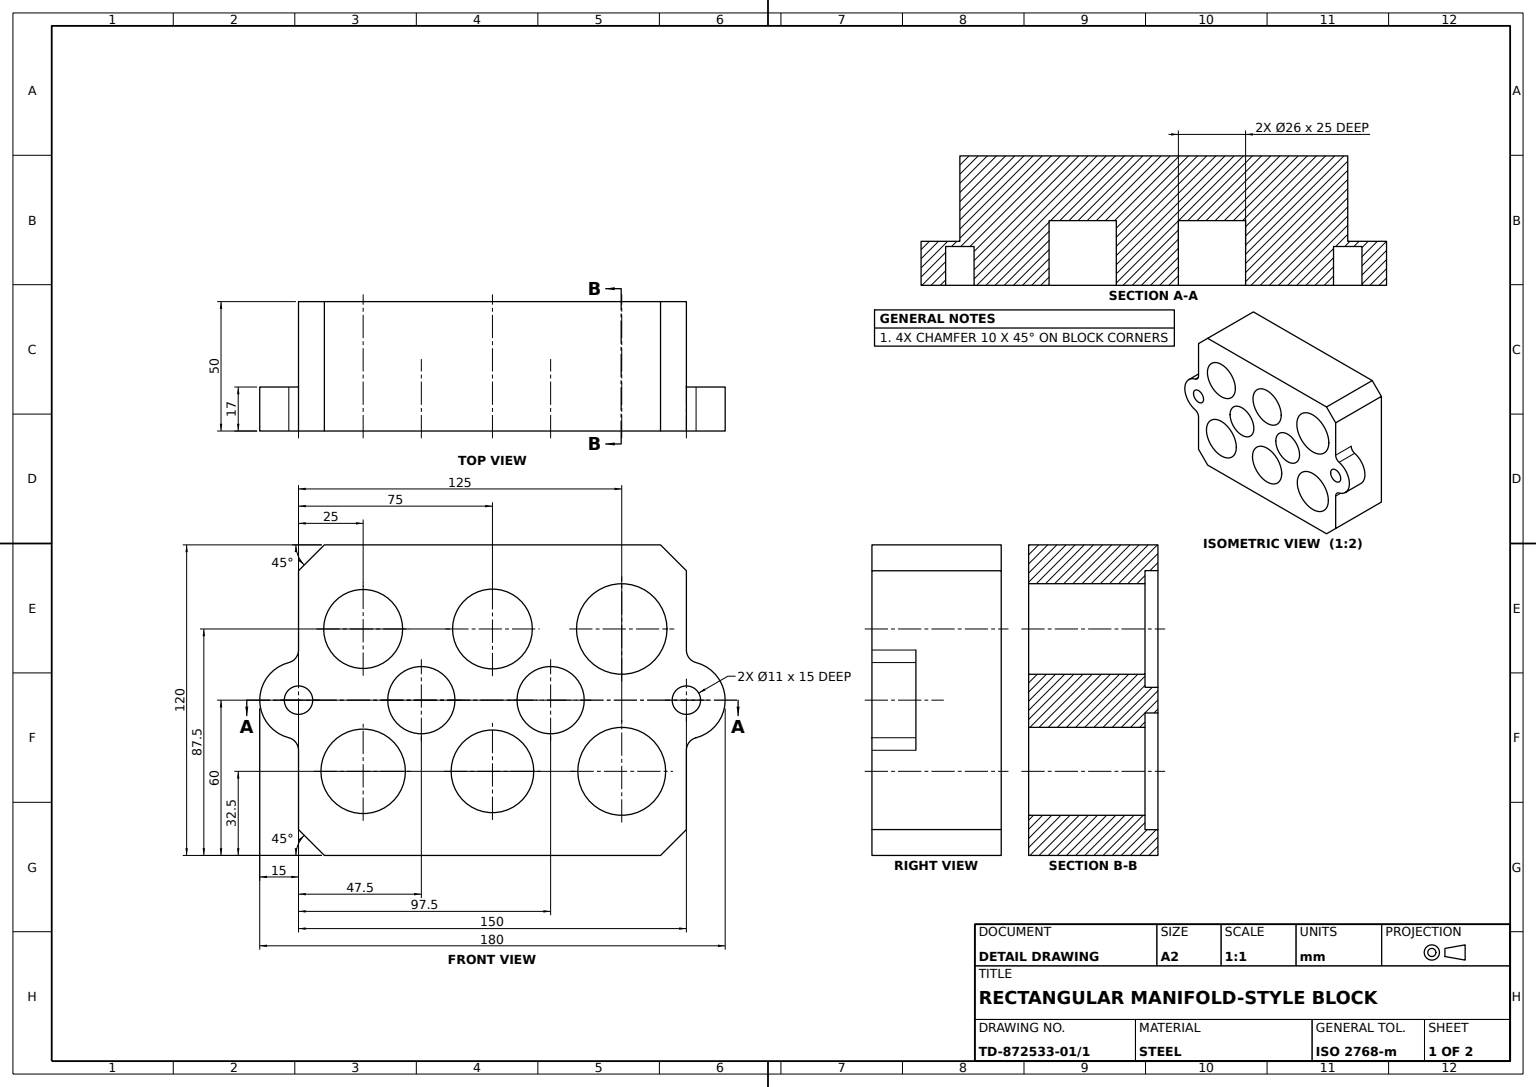
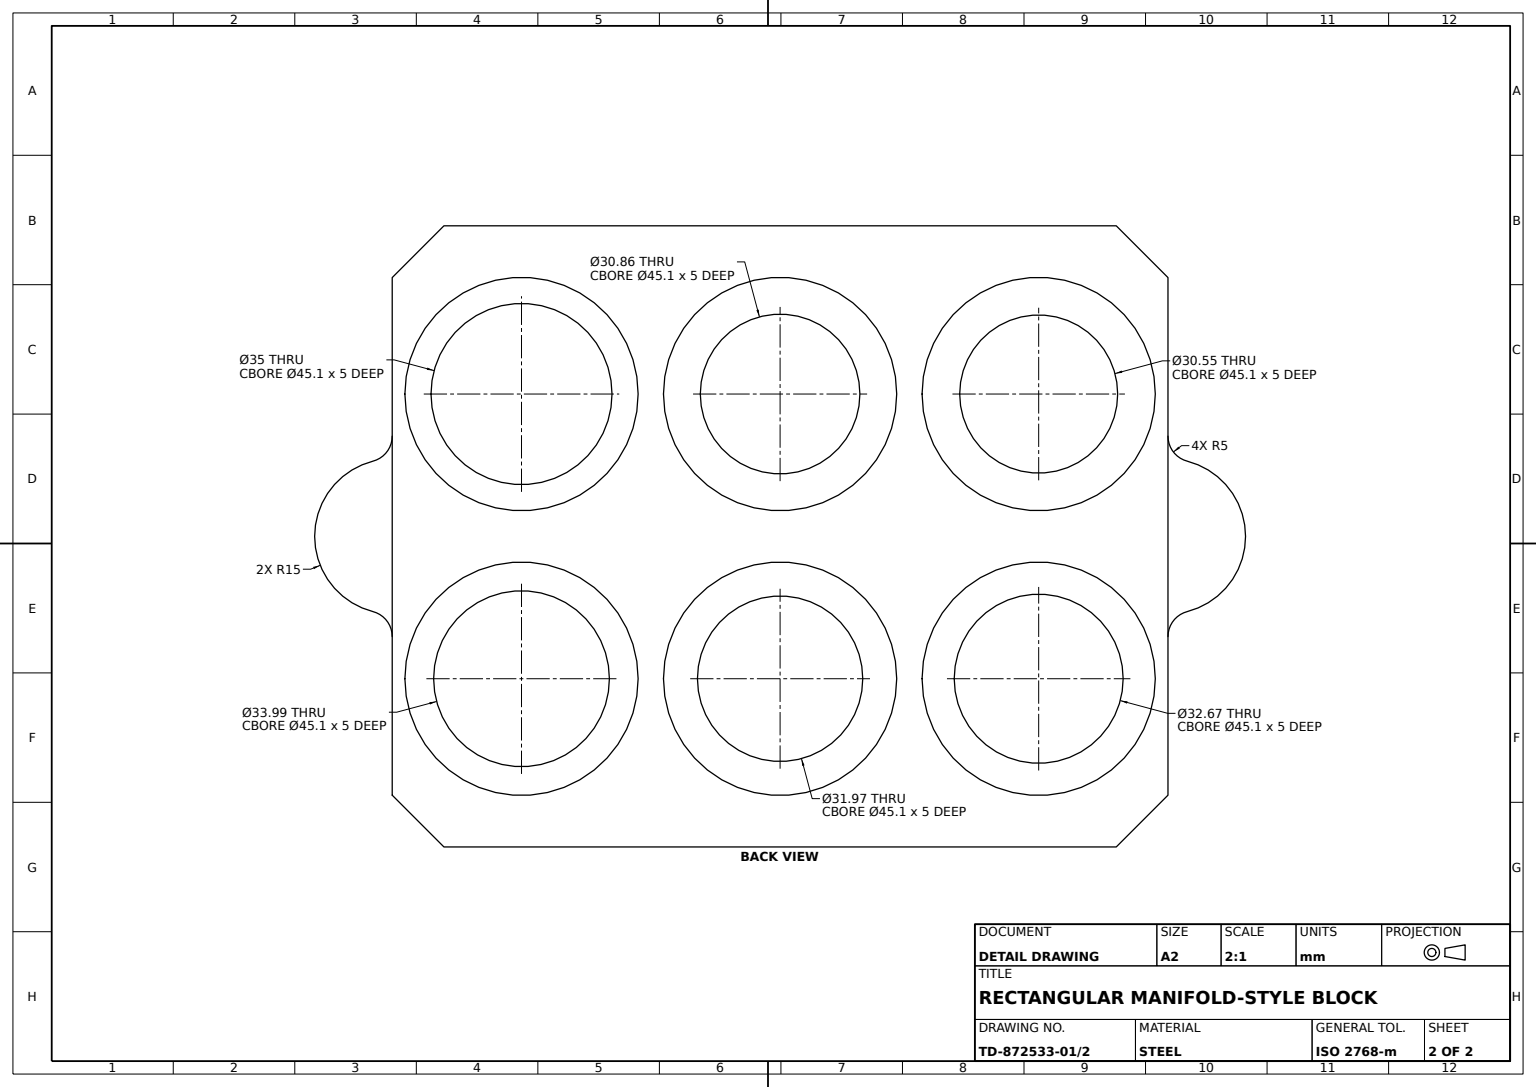
from build123d import *

# Parameters (mm, degrees)
BLOCK_PROFILE_SKETCH_W         = 150
BLOCK_PROFILE_SKETCH_H         = 120
BASE_BLOCK_150X120X50_DEPTH    = 50
PORT_COUNTERBORE_SKETCH_R      = 22.55
PORT_COUNTERBORES_5_DEEP_DEPTH = 5
PORT_HOLE_SKETCH_R             = 17.5
PORT_HOLE_SKETCH_R_2           = 15.429011377
PORT_HOLE_SKETCH_R_3           = 15.274258873
PORT_HOLE_SKETCH_R_4           = 16.993106502
PORT_HOLE_SKETCH_R_5           = 15.982646342
PORT_HOLE_SKETCH_R_6           = 16.333623566
PORT_THROUGH_HOLES_DEPTH       = 198.294196569
EDGE_CHAMFER_10X45_A_SIZE      = 10
EDGE_CHAMFER_10X45_B_SIZE      = 10
MOUNTING_EARS_DEPTH            = 17
EAR_HOLE_SKETCH_R              = 5.5
EAR_HOLES_DEPTH                = 15
SIDE_RECESS_SKETCH_R           = 13
SIDE_RECESS_DEPTH              = 25


with BuildPart() as part:
    # Block Profile Sketch → Base Block 150x120x50 (new body)
    with BuildSketch(Plane.XY):
        with Locations((75, 60)):
            Rectangle(BLOCK_PROFILE_SKETCH_W, BLOCK_PROFILE_SKETCH_H)
    extrude(amount=BASE_BLOCK_150X120X50_DEPTH)

    # Port Counterbore Sketch → Port Counterbores 5 Deep (cut)
    with BuildSketch(Plane(origin=(0, 0, 0), x_dir=(-1, 0, 0), z_dir=(0, 0, -1))):
        with Locations((-125, 87.5)):
            Circle(PORT_COUNTERBORE_SKETCH_R)
        with Locations((-75, 87.5)):
            Circle(PORT_COUNTERBORE_SKETCH_R)
        with Locations((-25, 87.5)):
            Circle(PORT_COUNTERBORE_SKETCH_R)
        with Locations((-25, 32.5)):
            Circle(PORT_COUNTERBORE_SKETCH_R)
        with Locations((-75, 32.5)):
            Circle(PORT_COUNTERBORE_SKETCH_R)
        with Locations((-125, 32.5)):
            Circle(PORT_COUNTERBORE_SKETCH_R)
    extrude(amount=-PORT_COUNTERBORES_5_DEEP_DEPTH, mode=Mode.SUBTRACT)

    # Port Hole Sketch → Port Through Holes (cut, through all)
    with BuildSketch(Plane(origin=(0, 0, 5), x_dir=(-1, 0, 0), z_dir=(0, 0, -1))):
        with Locations((-125, 87.5)):
            Circle(PORT_HOLE_SKETCH_R)
        with Locations((-75, 87.5)):
            Circle(PORT_HOLE_SKETCH_R_2)
        with Locations((-25, 87.5)):
            Circle(PORT_HOLE_SKETCH_R_3)
        with Locations((-125, 32.5)):
            Circle(PORT_HOLE_SKETCH_R_4)
        with Locations((-75, 32.5)):
            Circle(PORT_HOLE_SKETCH_R_5)
        with Locations((-25, 32.5)):
            Circle(PORT_HOLE_SKETCH_R_6)
    extrude(amount=-PORT_THROUGH_HOLES_DEPTH, mode=Mode.SUBTRACT)

    # Edge Chamfer 10x45 A
    edge_chamfer_10x45_a_edges = [part.edges().sort_by_distance(p)[0] for p in [
        (0, 0, 25),
    ]]
    chamfer(edge_chamfer_10x45_a_edges, length=EDGE_CHAMFER_10X45_A_SIZE)

    # Edge Chamfer 10x45 B
    edge_chamfer_10x45_b_edges = [part.edges().sort_by_distance(p)[0] for p in [
        (0, 120, 25),
        (150, 120, 25),
        (150, 0, 25),
    ]]
    chamfer(edge_chamfer_10x45_b_edges, length=EDGE_CHAMFER_10X45_B_SIZE)

    # Mounting Ear Profile Sketch → Mounting Ears (add)
    with BuildSketch(Plane.XY.offset(50)):
        with BuildLine():
            Line((0, 79.364916731), (0, 40.635083269))
            ThreePointArc((0, 40.635083269), (-1.047152925, 43.696945447), (-3.75, 45.476312452))
            ThreePointArc((-3.75, 45.476312452), (-15, 60), (-3.75, 74.523687548))
            ThreePointArc((-3.75, 74.523687548), (-1.047152925, 76.303054553), (0, 79.364916731))
        make_face()
        with BuildLine():
            Line((150, 79.364916731), (150, 40.635083269))
            ThreePointArc((150, 40.635083269), (151.047152925, 43.696945447), (153.75, 45.476312452))
            ThreePointArc((153.75, 45.476312452), (165, 60), (153.75, 74.523687548))
            ThreePointArc((153.75, 74.523687548), (151.047152925, 76.303054553), (150, 79.364916731))
        make_face()
    extrude(amount=-MOUNTING_EARS_DEPTH)

    # Ear Hole Sketch → Ear Holes (cut)
    with BuildSketch(Plane.XY.offset(50)):
        with Locations((150, 60)):
            Circle(EAR_HOLE_SKETCH_R)
        with Locations((0, 60)):
            Circle(EAR_HOLE_SKETCH_R)
    extrude(amount=-EAR_HOLES_DEPTH, mode=Mode.SUBTRACT)

    # Side Recess Sketch → Side Recess (cut)
    with BuildSketch(Plane.XY.offset(50)):
        with Locations((47.5, 60)):
            Circle(SIDE_RECESS_SKETCH_R)
        with Locations((97.5, 60)):
            Circle(SIDE_RECESS_SKETCH_R)
    extrude(amount=-SIDE_RECESS_DEPTH, mode=Mode.SUBTRACT)


solid = part.part
